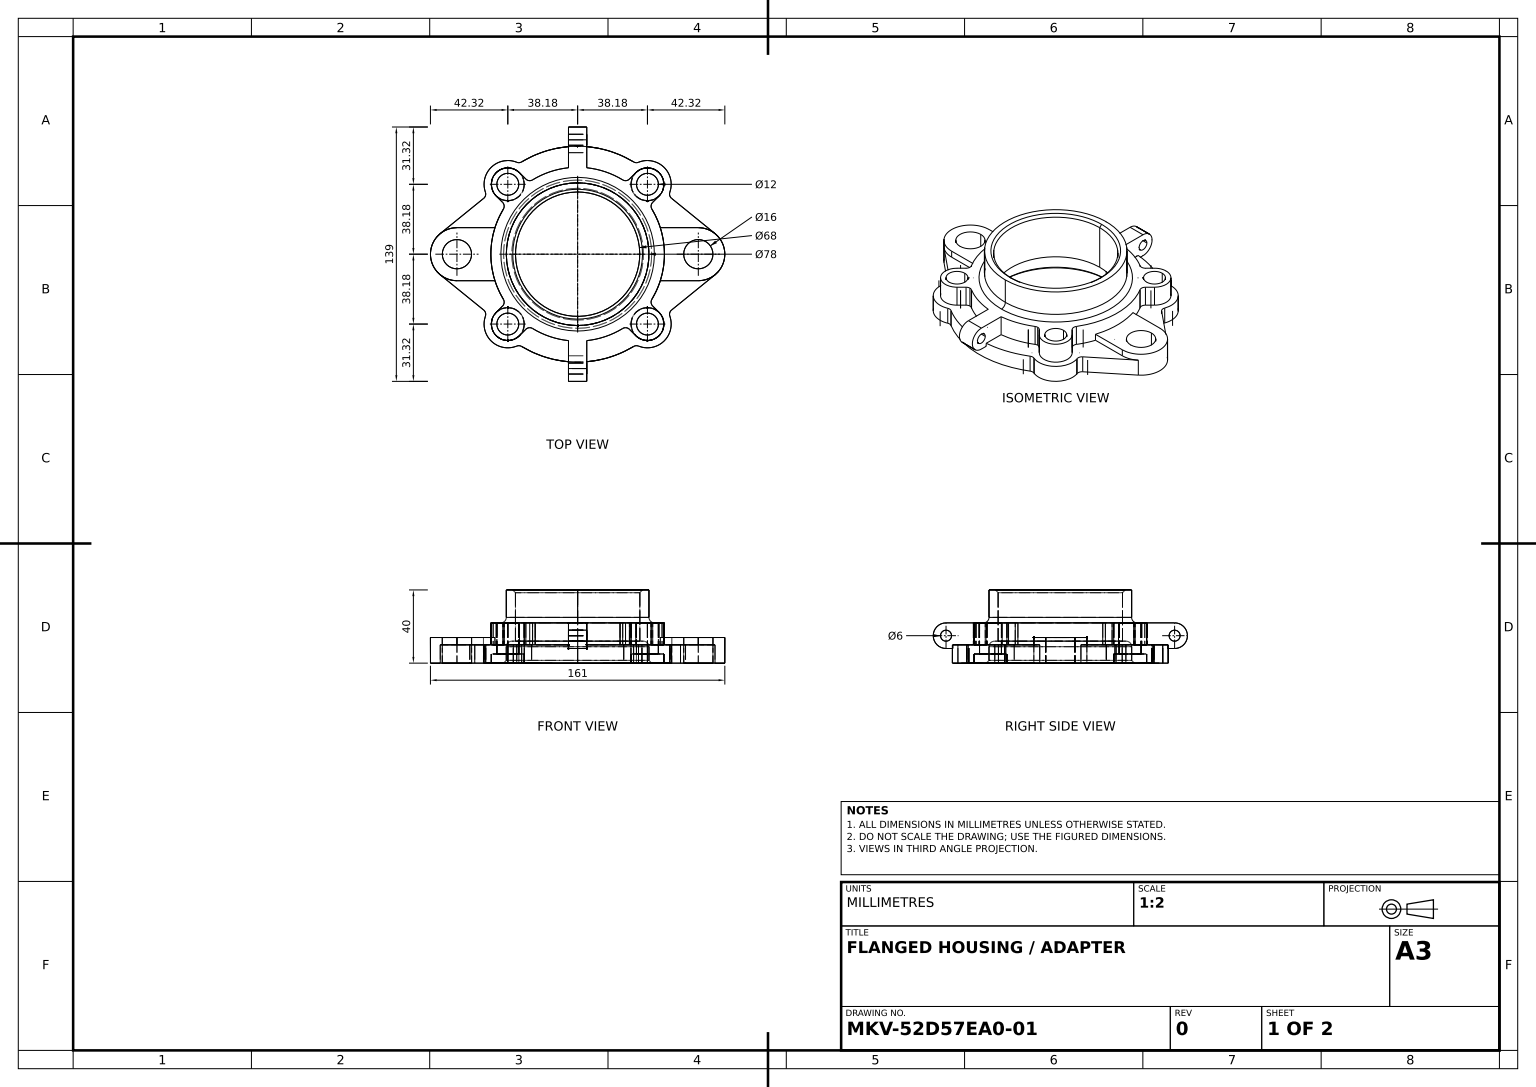
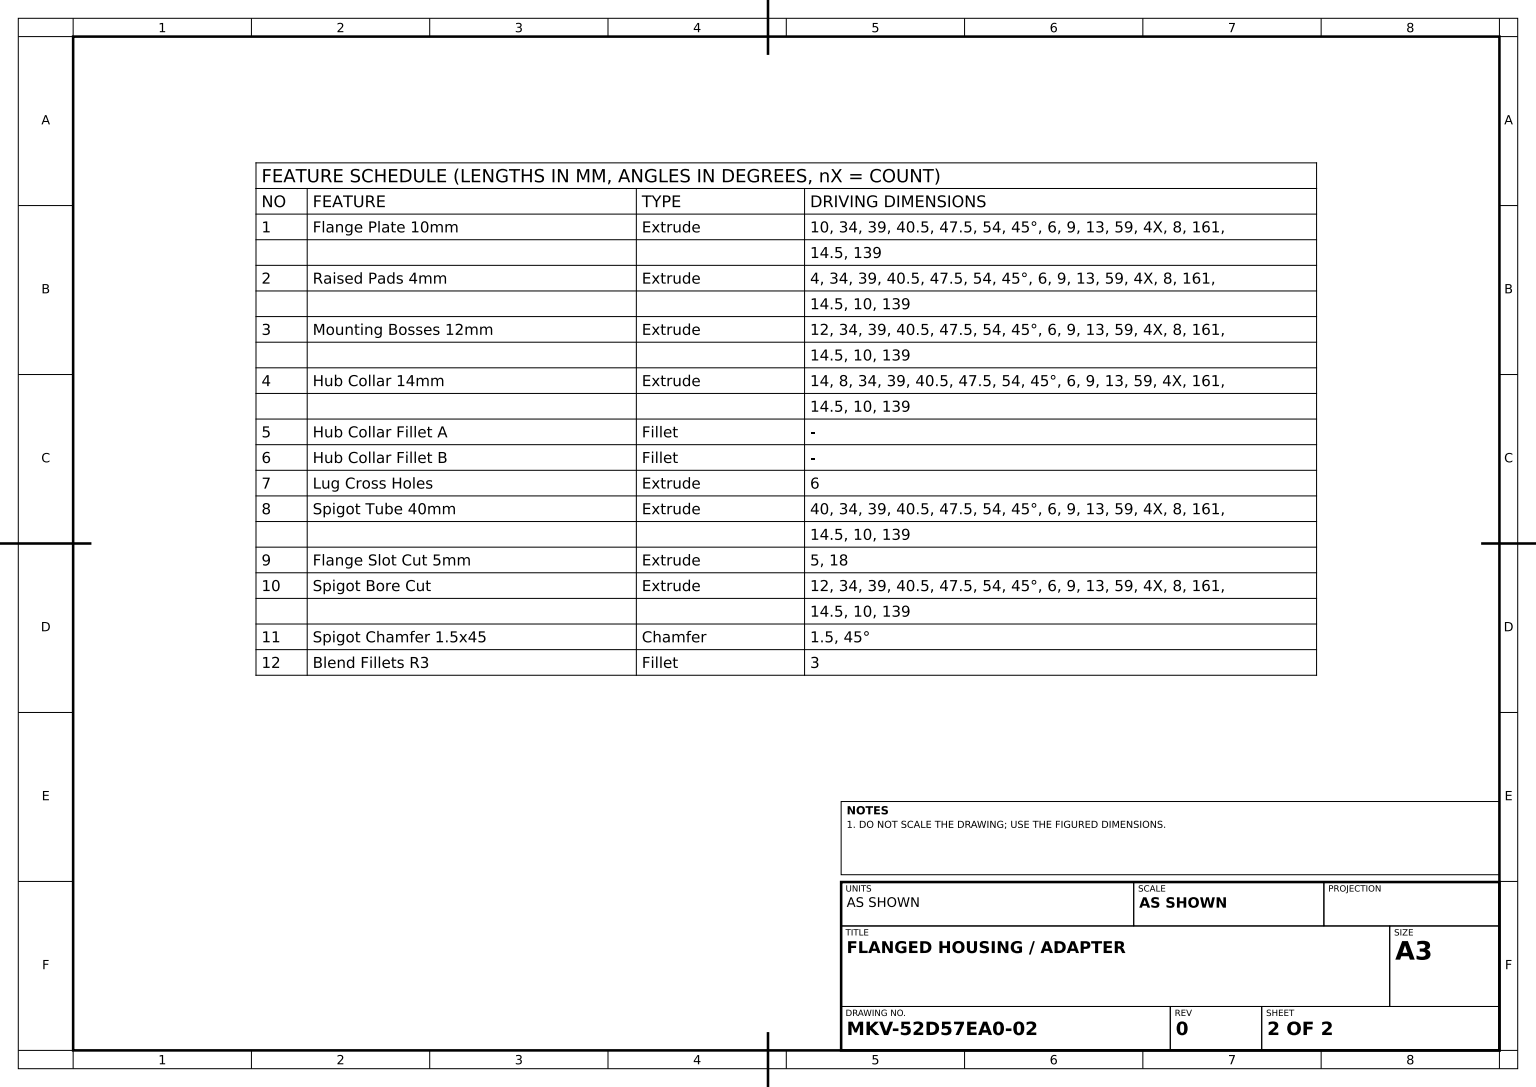
from build123d import *

# Parameters (mm, degrees)
HOUSING_MASTER_SKETCH_R        = 6
HOUSING_MASTER_SKETCH_R_2      = 39
HOUSING_MASTER_SKETCH_R_3      = 8
FLANGE_PLATE_10MM_DEPTH        = 10
RAISED_START                   = 10
SKETCH1_3_R                    = 8
RAISED_PADS_4MM_DEPTH          = 4
MOUNTING_START                 = 10
SKETCH1_4_R                    = 39
SKETCH1_4_R_2                  = 6
MOUNTING_BOSSES_12MM_DEPTH     = 12
HUB_START                      = 8
HUB_COLLAR_14MM_DEPTH          = 14
HUB_COLLAR_FILLET_A_RADIUS     = 7
HUB_COLLAR_FILLET_A_LENGTH     = 10
HUB_COLLAR_FILLET_B_RADIUS     = 7
HUB_COLLAR_FILLET_B_LENGTH     = 10
LUG_CROSS_HOLES_DEPTH          = 109.602486159
LUG_CROSS_HOLES_DEPTH_BACK     = 109.602486159
LUG_CROSS_HOLE_SKETCH_R        = 3
SKETCH1_7_R                    = 39
SKETCH1_7_R_2                  = 34
SPIGOT_TUBE_40MM_DEPTH         = 40
FLANGE_SLOT_CUT_5MM_DEPTH      = 114.624381186
FLANGE_SLOT_CUT_5MM_DEPTH_BACK = 5
FLANGE_SLOT_SKETCH_R           = 9
SKETCH1_9_R                    = 39
SKETCH1_9_R_2                  = 34
SPIGOT_BORE_CUT_DEPTH          = 12
SPIGOT_CHAMFER_1_5X45_SIZE     = 1.5
BLEND_FILLETS_R3_R             = 3


with BuildPart() as part:
    # Housing Master Sketch → Flange Plate 10mm (new body)
    with BuildSketch(Plane(origin=(0, 0, 0), x_dir=(1, 0, 0), z_dir=(0, 1, 0))):
        with BuildLine():
            Line((75.129231708, 11.265306406), (49.595662085, 31.957320012))
            ThreePointArc((49.595662085, 31.957320012), (47.376154339, 47.376154339), (31.957320012, 49.595662085))
            ThreePointArc((31.957320012, 49.595662085), (0, 59), (-31.957320012, 49.595662085))
            ThreePointArc((-31.957320012, 49.595662085), (-47.376154339, 47.376154339), (-49.595662085, 31.957320012))
            Line((-49.595662085, 31.957320012), (-75.129231708, 11.265306406))
            ThreePointArc((-75.129231708, 11.265306406), (-80.5, 0), (-75.129231708, -11.265306406))
            Line((-75.129231708, -11.265306406), (-49.595662085, -31.957320012))
            ThreePointArc((-49.595662085, -31.957320012), (-47.376154339, -47.376154339), (-31.957320012, -49.595662085))
            ThreePointArc((-31.957320012, -49.595662085), (0, -59), (31.957320012, -49.595662085))
            ThreePointArc((31.957320012, -49.595662085), (47.376154339, -47.376154339), (49.595662085, -31.957320012))
            Line((49.595662085, -31.957320012), (75.129231708, -11.265306406))
            ThreePointArc((75.129231708, -11.265306406), (80.5, 0), (75.129231708, 11.265306406))
        make_face()
        with Locations(Location((-38.183766184, -38.183766184, 0), (0, 0, 270))):
            Circle(HOUSING_MASTER_SKETCH_R, mode=Mode.SUBTRACT)
        with Locations(Location((38.183766184, -38.183766184, 0), (0, 0, 270))):
            Circle(HOUSING_MASTER_SKETCH_R, mode=Mode.SUBTRACT)
        with Locations(Location((0, 0, 0), (0, 0, 270))):
            Circle(HOUSING_MASTER_SKETCH_R_2, mode=Mode.SUBTRACT)
        with Locations(Location((-38.183766184, 38.183766184, 0), (0, 0, 270))):
            Circle(HOUSING_MASTER_SKETCH_R, mode=Mode.SUBTRACT)
        with Locations(Location((38.183766184, 38.183766184, 0), (0, 0, 270))):
            Circle(HOUSING_MASTER_SKETCH_R, mode=Mode.SUBTRACT)
        with Locations(Location((66, 0, 0), (0, 0, 270))):
            Circle(HOUSING_MASTER_SKETCH_R_3, mode=Mode.SUBTRACT)
        with Locations(Location((-66, 0, 0), (0, 0, 270))):
            Circle(HOUSING_MASTER_SKETCH_R_3, mode=Mode.SUBTRACT)
    extrude(amount=FLANGE_PLATE_10MM_DEPTH)

    # Sketch1_3 → Raised Pads 4mm (add)
    # profile 1 of 2: a face of its own
    with BuildSketch(Plane(origin=(0, 0, 0), x_dir=(1, 0, 0), z_dir=(0, 1, 0)).offset(RAISED_START)):
        with BuildLine():
            ThreePointArc((-66, 14.5), (-70.842677829, 13.667423731), (-75.129231708, 11.265306406))
            ThreePointArc((-75.129231708, 11.265306406), (-80.5, 0), (-75.129231708, -11.265306406))
            ThreePointArc((-75.129231708, -11.265306406), (-70.842677829, -13.667423731), (-66, -14.5))
            Line((-66, -14.5), (-45.232731512, -14.5))
            ThreePointArc((-45.232731512, -14.5), (-47.5, 0), (-45.232731512, 14.5))
            Line((-45.232731512, 14.5), (-66, 14.5))
        make_face()
        with Locations(Location((-66, 0, 0), (0, 0, 270))):
            Circle(SKETCH1_3_R, mode=Mode.SUBTRACT)
    # profile 2 of 2: a face of its own
    with BuildSketch(Plane(origin=(0, 0, 0), x_dir=(1, 0, 0), z_dir=(0, 1, 0)).offset(RAISED_START)):
        with BuildLine():
            Line((66, 14.5), (45.232731512, 14.5))
            ThreePointArc((45.232731512, 14.5), (47.5, 0), (45.232731512, -14.5))
            Line((45.232731512, -14.5), (66, -14.5))
            ThreePointArc((66, -14.5), (70.842677829, -13.667423731), (75.129231708, -11.265306406))
            ThreePointArc((75.129231708, -11.265306406), (80.5, 0), (75.129231708, 11.265306406))
            ThreePointArc((75.129231708, 11.265306406), (70.842677829, 13.667423731), (66, 14.5))
        make_face()
        with Locations(Location((66, 0, 0), (0, 0, 270))):
            Circle(SKETCH1_3_R, mode=Mode.SUBTRACT)
    extrude(amount=RAISED_PADS_4MM_DEPTH)



with BuildPart() as body_2:
    # Sketch1_4 → Mounting Bosses 12mm (new body)
    with BuildSketch(Plane(origin=(0, 0, 0), x_dir=(1, 0, 0), z_dir=(0, 1, 0)).offset(MOUNTING_START)):
        with BuildLine():
            Line((39.343121117, 26.615199056), (44.547727215, 31.819805153))
            ThreePointArc((44.547727215, 31.819805153), (44.547727215, 44.547727215), (31.819805153, 44.547727215))
            Line((31.819805153, 44.547727215), (26.615199056, 39.343121117))
            ThreePointArc((26.615199056, 39.343121117), (13.91854423, 45.415020935), (0, 47.5))
            ThreePointArc((0, 47.5), (-13.91854423, 45.415020935), (-26.615199056, 39.343121117))
            Line((-26.615199056, 39.343121117), (-31.819805153, 44.547727215))
            ThreePointArc((-31.819805153, 44.547727215), (-44.547727215, 44.547727215), (-44.547727215, 31.819805153))
            Line((-44.547727215, 31.819805153), (-39.343121117, 26.615199056))
            ThreePointArc((-39.343121117, 26.615199056), (-47.5, 0), (-39.343121117, -26.615199056))
            Line((-39.343121117, -26.615199056), (-44.547727215, -31.819805153))
            ThreePointArc((-44.547727215, -31.819805153), (-44.547727215, -44.547727215), (-31.819805153, -44.547727215))
            Line((-31.819805153, -44.547727215), (-26.615199056, -39.343121117))
            ThreePointArc((-26.615199056, -39.343121117), (-16.292790354, -44.618325635), (-5, -47.236109069))
            ThreePointArc((-5, -47.236109069), (11.505608296, -46.085474694), (26.615199056, -39.343121117))
            Line((26.615199056, -39.343121117), (31.819805153, -44.547727215))
            ThreePointArc((31.819805153, -44.547727215), (44.547727215, -44.547727215), (44.547727215, -31.819805153))
            Line((44.547727215, -31.819805153), (39.343121117, -26.615199056))
            ThreePointArc((39.343121117, -26.615199056), (47.5, 0), (39.343121117, 26.615199056))
        make_face()
        with Locations(Location((0, 0, 0), (0, 0, 270))):
            Circle(SKETCH1_4_R, mode=Mode.SUBTRACT)
        with Locations(Location((38.183766184, 38.183766184, 0), (0, 0, 270))):
            Circle(SKETCH1_4_R_2, mode=Mode.SUBTRACT)
        with Locations(Location((38.183766184, -38.183766184, 0), (0, 0, 270))):
            Circle(SKETCH1_4_R_2, mode=Mode.SUBTRACT)
        with Locations(Location((-38.183766184, -38.183766184, 0), (0, 0, 270))):
            Circle(SKETCH1_4_R_2, mode=Mode.SUBTRACT)
        with Locations(Location((-38.183766184, 38.183766184, 0), (0, 0, 270))):
            Circle(SKETCH1_4_R_2, mode=Mode.SUBTRACT)
    extrude(amount=MOUNTING_BOSSES_12MM_DEPTH)


with BuildPart() as part_1:
    add(part.part)

    add(body_2.part)  # Hub Collar 14mm merges body 2
    # Sketch1_6 → Hub Collar 14mm (add)
    with BuildSketch(Plane(origin=(0, 0, 0), x_dir=(1, 0, 0), z_dir=(0, 1, 0)).offset(HUB_START)):
        with BuildLine():
            Line((5, 47.236109069), (5, 69.5))
            Line((5, 69.5), (-5, 69.5))
            Line((-5, 69.5), (-5, 47.236109069))
            ThreePointArc((-5, 47.236109069), (0, 47.5), (5, 47.236109069))
        make_face()
        with BuildLine():
            Line((-5, -47.236109069), (-5, -69.5))
            Line((-5, -69.5), (5, -69.5))
            Line((5, -69.5), (5, -47.236109069))
            ThreePointArc((5, -47.236109069), (0, -47.5), (-5, -47.236109069))
        make_face()
    extrude(amount=HUB_COLLAR_14MM_DEPTH)

    # Hub Collar Fillet A: full round fillet: the end face becomes a half cylinder, R = half its width
    hub_collar_fillet_a_face = Plane((0, 15, 69.5), x_dir=(1, 0, 0), z_dir=(0, 0, 1))  # on the end face: x along it, z out of the body
    hub_collar_fillet_a_slab = hub_collar_fillet_a_face.offset(-HUB_COLLAR_FILLET_A_RADIUS / 2) * Box(HUB_COLLAR_FILLET_A_LENGTH, 2 * HUB_COLLAR_FILLET_A_RADIUS, HUB_COLLAR_FILLET_A_RADIUS, mode=Mode.PRIVATE)  # the body's end, R deep
    hub_collar_fillet_a_round = Plane((0, 15, 62.5), x_dir=(0, 0, 1), z_dir=(1, 0, 0)) * Cylinder(HUB_COLLAR_FILLET_A_RADIUS, HUB_COLLAR_FILLET_A_LENGTH, mode=Mode.PRIVATE)  # its axis R under the face
    add(hub_collar_fillet_a_slab - hub_collar_fillet_a_round, mode=Mode.SUBTRACT)

    # Hub Collar Fillet B: full round fillet: the end face becomes a half cylinder, R = half its width
    hub_collar_fillet_b_face = Plane((0, 15, -69.5), x_dir=(1, 0, 0), z_dir=(0, 0, -1))  # on the end face: x along it, z out of the body
    hub_collar_fillet_b_slab = hub_collar_fillet_b_face.offset(-HUB_COLLAR_FILLET_B_RADIUS / 2) * Box(HUB_COLLAR_FILLET_B_LENGTH, 2 * HUB_COLLAR_FILLET_B_RADIUS, HUB_COLLAR_FILLET_B_RADIUS, mode=Mode.PRIVATE)  # the body's end, R deep
    hub_collar_fillet_b_round = Plane((0, 15, -62.5), x_dir=(0, 0, -1), z_dir=(1, 0, 0)) * Cylinder(HUB_COLLAR_FILLET_B_RADIUS, HUB_COLLAR_FILLET_B_LENGTH, mode=Mode.PRIVATE)  # its axis R under the face
    add(hub_collar_fillet_b_slab - hub_collar_fillet_b_round, mode=Mode.SUBTRACT)

    # Lug Cross Hole Sketch → Lug Cross Holes (cut, two sides: drawn at the far end of the back side and taken through both)
    with BuildSketch(Plane(origin=(0, 0, 0), x_dir=(0, 0, -1), z_dir=(1, 0, 0)).offset(-LUG_CROSS_HOLES_DEPTH_BACK)):
        with Locations((-62.5, 15)):
            Circle(LUG_CROSS_HOLE_SKETCH_R)
        with Locations(Location((62.5, 15, 0), (0, 0, 180))):
            Circle(LUG_CROSS_HOLE_SKETCH_R)
    extrude(amount=LUG_CROSS_HOLES_DEPTH + LUG_CROSS_HOLES_DEPTH_BACK, mode=Mode.SUBTRACT)

    # Sketch1_7 → Spigot Tube 40mm (add)
    with BuildSketch(Plane(origin=(0, 0, 0), x_dir=(1, 0, 0), z_dir=(0, 1, 0))):
        with Locations(Location((0, 0, 0), (0, 0, 270))):
            Circle(SKETCH1_7_R)
        with Locations(Location((0, 0, 0), (0, 0, 270))):
            Circle(SKETCH1_7_R_2, mode=Mode.SUBTRACT)
    extrude(amount=SPIGOT_TUBE_40MM_DEPTH)

    # Flange Slot Sketch → Flange Slot Cut 5mm (cut, two sides: drawn at the far end of the back side and taken through both)
    with BuildSketch(Plane.XZ.offset(-FLANGE_SLOT_CUT_5MM_DEPTH_BACK)):
        with Locations(Location((-38.183766184, 38.183766184, 0), (0, 0, 270))):
            Circle(FLANGE_SLOT_SKETCH_R)
        with Locations(Location((38.183766184, 38.183766184, 0), (0, 0, 270))):
            Circle(FLANGE_SLOT_SKETCH_R)
        with Locations(Location((38.183766184, -38.183766184, 0), (0, 0, 270))):
            Circle(FLANGE_SLOT_SKETCH_R)
        with Locations(Location((-38.183766184, -38.183766184, 0), (0, 0, 270))):
            Circle(FLANGE_SLOT_SKETCH_R)
    extrude(amount=FLANGE_SLOT_CUT_5MM_DEPTH + FLANGE_SLOT_CUT_5MM_DEPTH_BACK, mode=Mode.SUBTRACT)

    # Sketch1_9 → Spigot Bore Cut (cut)
    with BuildSketch(Plane(origin=(0, 0, 0), x_dir=(1, 0, 0), z_dir=(0, 1, 0))):
        with Locations(Location((0, 0, 0), (0, 0, 270))):
            Circle(SKETCH1_9_R)
        with Locations(Location((0, 0, 0), (0, 0, 270))):
            Circle(SKETCH1_9_R_2, mode=Mode.SUBTRACT)
    extrude(amount=SPIGOT_BORE_CUT_DEPTH, mode=Mode.SUBTRACT)

    # Spigot Chamfer 1.5x45
    spigot_chamfer_1_5x45_edges = [part_1.edges().sort_by_distance(p)[0] for p in [
        (0, 40, -34),
        (0, 0, -39),
    ]]
    chamfer(spigot_chamfer_1_5x45_edges, length=SPIGOT_CHAMFER_1_5X45_SIZE)

    # Blend Fillets R3
    blend_fillets_r3_edges = [part_1.edges().sort_by_distance(p)[0] for p in [
        (-26.615199056, 16, 39.343121117),
        (26.615199056, 16, 39.343121117),
        (39.343121117, 16, 26.615199056),
        (39.343121117, 16, -26.615199056),
        (26.615199056, 16, -39.343121117),
        (-26.615199056, 16, -39.343121117),
        (-39.343121117, 16, -26.615199056),
        (-39.343121117, 16, 26.615199056),
        (0, 22, -39),
        (0, 12, -39),
        (49.595662085, 5, 31.957320012),
        (31.957320012, 5, 49.595662085),
        (-31.957320012, 5, 49.595662085),
        (-49.595662085, 5, 31.957320012),
        (-49.595662085, 5, -31.957320012),
        (-31.957320012, 5, -49.595662085),
        (31.957320012, 5, -49.595662085),
        (49.595662085, 5, -31.957320012),
    ]]
    fillet(blend_fillets_r3_edges, radius=BLEND_FILLETS_R3_R)


solid = part_1.part
